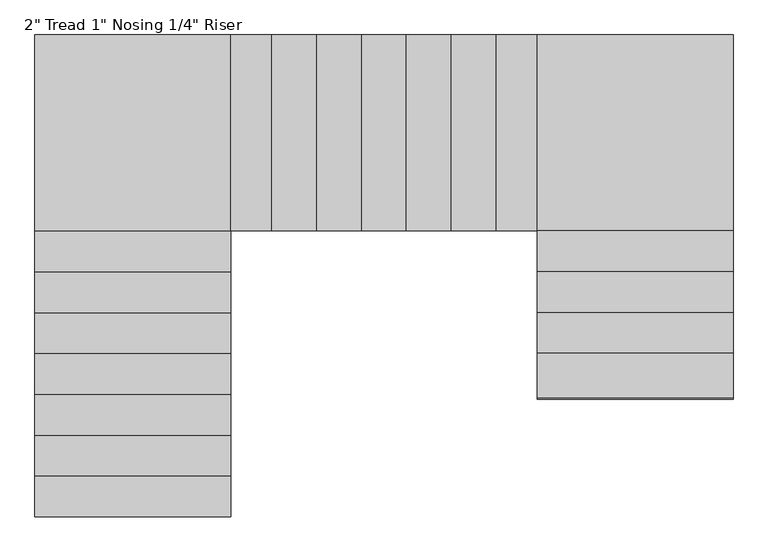
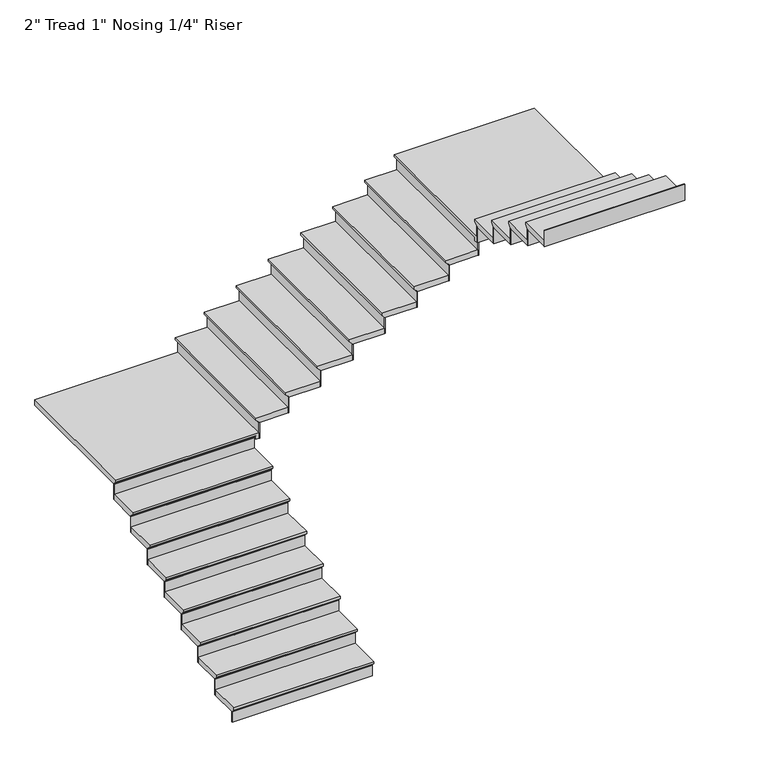
"""IFC4 building model written with IfcOpenShell, lengths in millimetres: stair flight geometry."""

from ifc_helpers import new_model, si_unit, origin, place, context, project, spatial, faceted_brep, source, transform, mapped, element, save


def stair_flight_18be0a75(model_context):
    return source(origin(), model_context, "Body", "Brep", [
        faceted_brep([(14512.1100959, 14647.8480703, 126.0928571), (14512.1100959, 14647.8480703, 145.1428571), (13292.9100959, 14647.8480703, 145.1428571), (13292.9100959, 14647.8480703, 126.0928571), (14512.1100959, 14673.2480703, 100.6928571), (13292.9100959, 14673.2480703, 100.6928571), (14512.1100959, 14927.2480703, 145.1428571), (13292.9100959, 14927.2480703, 145.1428571), (13292.9100959, 14673.2480703, 94.3428571), (13292.9100959, 14927.2480703, 94.3428571), (14512.1100959, 14927.2480703, 94.3428571), (14512.1100959, 14673.2480703, 94.3428571)], [[[0, 1, 2, 3]], [[4, 0, 3, 5]], [[2, 1, 6, 7]], [[8, 9, 10, 11]], [[2, 7, 9, 8, 5, 3]], [[8, 11, 4, 5]], [[6, 1, 0, 4, 11, 10]], [[7, 6, 10, 9]]]),
        faceted_brep([(14512.1100959, 14673.2480703, 94.3428571), (14512.1100959, 14673.2480703, 0.0), (14512.1100959, 14679.5980703, 0.0), (14512.1100959, 14679.5980703, 94.3428571), (13292.9100959, 14673.2480703, 94.3428571), (13292.9100959, 14679.5980703, 94.3428571), (13292.9100959, 14679.5980703, 0.0), (13292.9100959, 14673.2480703, 0.0)], [[[0, 1, 2, 3]], [[4, 5, 6, 7]], [[1, 0, 4, 7]], [[2, 1, 7, 6]], [[3, 2, 6, 5]], [[0, 3, 5, 4]]]),
        faceted_brep([(14512.1100959, 14927.2480703, 239.4857143), (14512.1100959, 14927.2480703, 94.3428571), (14512.1100959, 14933.5980703, 94.3428571), (14512.1100959, 14933.5980703, 239.4857143), (13292.9100959, 14927.2480703, 239.4857143), (13292.9100959, 14933.5980703, 239.4857143), (13292.9100959, 14933.5980703, 94.3428571), (13292.9100959, 14927.2480703, 94.3428571)], [[[0, 1, 2, 3]], [[4, 5, 6, 7]], [[1, 0, 4, 7]], [[2, 1, 7, 6]], [[3, 2, 6, 5]], [[0, 3, 5, 4]]]),
        faceted_brep([(13292.9100959, 14901.8480703, 290.2857143), (14512.1100959, 14901.8480703, 290.2857143), (14512.1100959, 15181.2480703, 290.2857143), (13292.9100959, 15181.2480703, 290.2857143), (13292.9100959, 14927.2480703, 239.4857143), (13292.9100959, 15181.2480703, 239.4857143), (14512.1100959, 15181.2480703, 239.4857143), (14512.1100959, 14927.2480703, 239.4857143), (13292.9100959, 14927.2480703, 245.8357143), (13292.9100959, 14901.8480703, 271.2357143), (14512.1100959, 14927.2480703, 245.8357143), (14512.1100959, 14901.8480703, 271.2357143)], [[[0, 1, 2, 3]], [[4, 5, 6, 7]], [[0, 3, 5, 4, 8, 9]], [[4, 7, 10, 8]], [[2, 1, 11, 10, 7, 6]], [[3, 2, 6, 5]], [[11, 1, 0, 9]], [[10, 11, 9, 8]]]),
        faceted_brep([(14512.1100959, 15181.2480703, 384.6285714), (14512.1100959, 15181.2480703, 239.4857143), (14512.1100959, 15187.5980703, 239.4857143), (14512.1100959, 15187.5980703, 384.6285714), (13292.9100959, 15181.2480703, 384.6285714), (13292.9100959, 15187.5980703, 384.6285714), (13292.9100959, 15187.5980703, 239.4857143), (13292.9100959, 15181.2480703, 239.4857143)], [[[0, 1, 2, 3]], [[4, 5, 6, 7]], [[1, 0, 4, 7]], [[2, 1, 7, 6]], [[3, 2, 6, 5]], [[0, 3, 5, 4]]]),
        faceted_brep([(13292.9100959, 15155.8480703, 435.4285714), (14512.1100959, 15155.8480703, 435.4285714), (14512.1100959, 15435.2480703, 435.4285714), (13292.9100959, 15435.2480703, 435.4285714), (13292.9100959, 15181.2480703, 384.6285714), (13292.9100959, 15435.2480703, 384.6285714), (14512.1100959, 15435.2480703, 384.6285714), (14512.1100959, 15181.2480703, 384.6285714), (13292.9100959, 15181.2480703, 390.9785714), (13292.9100959, 15155.8480703, 416.3785714), (14512.1100959, 15181.2480703, 390.9785714), (14512.1100959, 15155.8480703, 416.3785714)], [[[0, 1, 2, 3]], [[4, 5, 6, 7]], [[0, 3, 5, 4, 8, 9]], [[4, 7, 10, 8]], [[2, 1, 11, 10, 7, 6]], [[3, 2, 6, 5]], [[11, 1, 0, 9]], [[10, 11, 9, 8]]]),
        faceted_brep([(14512.1100959, 15435.2480703, 529.7714286), (14512.1100959, 15435.2480703, 384.6285714), (14512.1100959, 15441.5980703, 384.6285714), (14512.1100959, 15441.5980703, 529.7714286), (13292.9100959, 15435.2480703, 529.7714286), (13292.9100959, 15441.5980703, 529.7714286), (13292.9100959, 15441.5980703, 384.6285714), (13292.9100959, 15435.2480703, 384.6285714)], [[[0, 1, 2, 3]], [[4, 5, 6, 7]], [[1, 0, 4, 7]], [[2, 1, 7, 6]], [[3, 2, 6, 5]], [[0, 3, 5, 4]]]),
        faceted_brep([(13292.9100959, 15409.8480703, 580.5714286), (14512.1100959, 15409.8480703, 580.5714286), (14512.1100959, 15689.2480703, 580.5714286), (13292.9100959, 15689.2480703, 580.5714286), (13292.9100959, 15435.2480703, 529.7714286), (13292.9100959, 15689.2480703, 529.7714286), (14512.1100959, 15689.2480703, 529.7714286), (14512.1100959, 15435.2480703, 529.7714286), (13292.9100959, 15435.2480703, 536.1214286), (13292.9100959, 15409.8480703, 561.5214286), (14512.1100959, 15435.2480703, 536.1214286), (14512.1100959, 15409.8480703, 561.5214286)], [[[0, 1, 2, 3]], [[4, 5, 6, 7]], [[0, 3, 5, 4, 8, 9]], [[4, 7, 10, 8]], [[2, 1, 11, 10, 7, 6]], [[3, 2, 6, 5]], [[11, 1, 0, 9]], [[10, 11, 9, 8]]]),
        faceted_brep([(14512.1100959, 15689.2480703, 674.9142857), (14512.1100959, 15689.2480703, 529.7714286), (14512.1100959, 15695.5980703, 529.7714286), (14512.1100959, 15695.5980703, 674.9142857), (13292.9100959, 15689.2480703, 674.9142857), (13292.9100959, 15695.5980703, 674.9142857), (13292.9100959, 15695.5980703, 529.7714286), (13292.9100959, 15689.2480703, 529.7714286)], [[[0, 1, 2, 3]], [[4, 5, 6, 7]], [[1, 0, 4, 7]], [[2, 1, 7, 6]], [[3, 2, 6, 5]], [[0, 3, 5, 4]]]),
        faceted_brep([(13292.9100959, 15663.8480703, 725.7142857), (14512.1100959, 15663.8480703, 725.7142857), (14512.1100959, 15943.2480703, 725.7142857), (13292.9100959, 15943.2480703, 725.7142857), (13292.9100959, 15689.2480703, 674.9142857), (13292.9100959, 15943.2480703, 674.9142857), (14512.1100959, 15943.2480703, 674.9142857), (14512.1100959, 15689.2480703, 674.9142857), (13292.9100959, 15689.2480703, 681.2642857), (13292.9100959, 15663.8480703, 706.6642857), (14512.1100959, 15689.2480703, 681.2642857), (14512.1100959, 15663.8480703, 706.6642857)], [[[0, 1, 2, 3]], [[4, 5, 6, 7]], [[0, 3, 5, 4, 8, 9]], [[4, 7, 10, 8]], [[2, 1, 11, 10, 7, 6]], [[3, 2, 6, 5]], [[11, 1, 0, 9]], [[10, 11, 9, 8]]]),
        faceted_brep([(14512.1100959, 15943.2480703, 820.0571429), (14512.1100959, 15943.2480703, 674.9142857), (14512.1100959, 15949.5980703, 674.9142857), (14512.1100959, 15949.5980703, 820.0571429), (13292.9100959, 15943.2480703, 820.0571429), (13292.9100959, 15949.5980703, 820.0571429), (13292.9100959, 15949.5980703, 674.9142857), (13292.9100959, 15943.2480703, 674.9142857)], [[[0, 1, 2, 3]], [[4, 5, 6, 7]], [[1, 0, 4, 7]], [[2, 1, 7, 6]], [[3, 2, 6, 5]], [[0, 3, 5, 4]]]),
        faceted_brep([(13292.9100959, 15917.8480703, 870.8571429), (14512.1100959, 15917.8480703, 870.8571429), (14512.1100959, 16197.2480703, 870.8571429), (13292.9100959, 16197.2480703, 870.8571429), (13292.9100959, 15943.2480703, 820.0571429), (13292.9100959, 16197.2480703, 820.0571429), (14512.1100959, 16197.2480703, 820.0571429), (14512.1100959, 15943.2480703, 820.0571429), (13292.9100959, 15943.2480703, 826.4071429), (13292.9100959, 15917.8480703, 851.8071429), (14512.1100959, 15943.2480703, 826.4071429), (14512.1100959, 15917.8480703, 851.8071429)], [[[0, 1, 2, 3]], [[4, 5, 6, 7]], [[0, 3, 5, 4, 8, 9]], [[4, 7, 10, 8]], [[2, 1, 11, 10, 7, 6]], [[3, 2, 6, 5]], [[11, 1, 0, 9]], [[10, 11, 9, 8]]]),
        faceted_brep([(14512.1100959, 16197.2480703, 965.2), (14512.1100959, 16197.2480703, 820.0571429), (14512.1100959, 16203.5980703, 820.0571429), (14512.1100959, 16203.5980703, 965.2), (13292.9100959, 16197.2480703, 965.2), (13292.9100959, 16203.5980703, 965.2), (13292.9100959, 16203.5980703, 820.0571429), (13292.9100959, 16197.2480703, 820.0571429)], [[[0, 1, 2, 3]], [[4, 5, 6, 7]], [[1, 0, 4, 7]], [[2, 1, 7, 6]], [[3, 2, 6, 5]], [[0, 3, 5, 4]]]),
        faceted_brep([(13292.9100959, 16171.8480703, 1016.0), (14512.1100959, 16171.8480703, 1016.0), (14512.1100959, 16451.2480703, 1016.0), (13292.9100959, 16451.2480703, 1016.0), (13292.9100959, 16197.2480703, 965.2), (13292.9100959, 16451.2480703, 965.2), (14512.1100959, 16451.2480703, 965.2), (14512.1100959, 16197.2480703, 965.2), (13292.9100959, 16197.2480703, 971.55), (13292.9100959, 16171.8480703, 996.95), (14512.1100959, 16197.2480703, 971.55), (14512.1100959, 16171.8480703, 996.95)], [[[0, 1, 2, 3]], [[4, 5, 6, 7]], [[0, 3, 5, 4, 8, 9]], [[4, 7, 10, 8]], [[2, 1, 11, 10, 7, 6]], [[3, 2, 6, 5]], [[11, 1, 0, 9]], [[10, 11, 9, 8]]]),
        faceted_brep([(14512.1100959, 16451.2480703, 1110.3428571), (14512.1100959, 16451.2480703, 965.2), (14512.1100959, 16457.5980703, 965.2), (14512.1100959, 16457.5980703, 1110.3428571), (13292.9100959, 16451.2480703, 1110.3428571), (13292.9100959, 16457.5980703, 1110.3428571), (13292.9100959, 16457.5980703, 965.2), (13292.9100959, 16451.2480703, 965.2)], [[[0, 1, 2, 3]], [[4, 5, 6, 7]], [[1, 0, 4, 7]], [[2, 1, 7, 6]], [[3, 2, 6, 5]], [[0, 3, 5, 4]]]),
        faceted_brep([(14537.5100959, 17645.0480703, 1161.1428571), (13292.9100959, 17645.0480703, 1161.1428571), (13292.9100959, 16425.8480703, 1161.1428571), (14537.5100959, 16425.8480703, 1161.1428571), (13292.9100959, 17645.0480703, 1110.3428571), (14537.5100959, 17645.0480703, 1110.3428571), (14537.5100959, 16425.8480703, 1110.3428571), (14512.1100959, 16425.8480703, 1110.3428571), (14512.1100959, 16451.2480703, 1110.3428571), (13292.9100959, 16451.2480703, 1110.3428571), (13292.9100959, 16451.2480703, 1116.6928571), (13292.9100959, 16425.8480703, 1142.0928571), (14512.1100959, 16451.2480703, 1116.6928571), (14512.1100959, 16425.8480703, 1142.0928571)], [[[0, 1, 2, 3]], [[4, 5, 6, 7, 8, 9]], [[1, 0, 5, 4]], [[2, 1, 4, 9, 10, 11]], [[9, 8, 12, 10]], [[8, 7, 13, 12]], [[3, 2, 11, 13, 7, 6]], [[0, 3, 6, 5]], [[11, 10, 12, 13]]]),
        faceted_brep([(14537.5100959, 16425.8480703, 1255.4857143), (14537.5100959, 16425.8480703, 1110.3428571), (14543.8600959, 16425.8480703, 1110.3428571), (14543.8600959, 16425.8480703, 1255.4857143), (14537.5100959, 17645.0480703, 1255.4857143), (14543.8600959, 17645.0480703, 1255.4857143), (14543.8600959, 17645.0480703, 1110.3428571), (14537.5100959, 17645.0480703, 1110.3428571)], [[[0, 1, 2, 3]], [[4, 5, 6, 7]], [[1, 0, 4, 7]], [[2, 1, 7, 6]], [[3, 2, 6, 5]], [[0, 3, 5, 4]]]),
        faceted_brep([(14512.1100959, 17645.0480703, 1306.2857143), (14512.1100959, 16425.8480703, 1306.2857143), (14791.5100959, 16425.8480703, 1306.2857143), (14791.5100959, 17645.0480703, 1306.2857143), (14537.5100959, 17645.0480703, 1255.4857143), (14791.5100959, 17645.0480703, 1255.4857143), (14791.5100959, 16425.8480703, 1255.4857143), (14537.5100959, 16425.8480703, 1255.4857143), (14537.5100959, 17645.0480703, 1261.8357143), (14512.1100959, 17645.0480703, 1287.2357143), (14537.5100959, 16425.8480703, 1261.8357143), (14512.1100959, 16425.8480703, 1287.2357143)], [[[0, 1, 2, 3]], [[4, 5, 6, 7]], [[0, 3, 5, 4, 8, 9]], [[4, 7, 10, 8]], [[2, 1, 11, 10, 7, 6]], [[3, 2, 6, 5]], [[11, 1, 0, 9]], [[10, 11, 9, 8]]]),
        faceted_brep([(14791.5100959, 16425.8480703, 1400.6285714), (14791.5100959, 16425.8480703, 1255.4857143), (14797.8600959, 16425.8480703, 1255.4857143), (14797.8600959, 16425.8480703, 1400.6285714), (14791.5100959, 17645.0480703, 1400.6285714), (14797.8600959, 17645.0480703, 1400.6285714), (14797.8600959, 17645.0480703, 1255.4857143), (14791.5100959, 17645.0480703, 1255.4857143)], [[[0, 1, 2, 3]], [[4, 5, 6, 7]], [[1, 0, 4, 7]], [[2, 1, 7, 6]], [[3, 2, 6, 5]], [[0, 3, 5, 4]]]),
        faceted_brep([(14766.1100959, 17645.0480703, 1451.4285714), (14766.1100959, 16425.8480703, 1451.4285714), (15070.9100959, 16425.8480703, 1451.4285714), (15070.9100959, 17645.0480703, 1451.4285714), (14791.5100959, 17645.0480703, 1400.6285714), (15070.9100959, 17645.0480703, 1400.6285714), (15070.9100959, 16425.8480703, 1400.6285714), (14791.5100959, 16425.8480703, 1400.6285714), (14791.5100959, 17645.0480703, 1406.9785714), (14766.1100959, 17645.0480703, 1432.3785714), (14791.5100959, 16425.8480703, 1406.9785714), (14766.1100959, 16425.8480703, 1432.3785714)], [[[0, 1, 2, 3]], [[4, 5, 6, 7]], [[0, 3, 5, 4, 8, 9]], [[4, 7, 10, 8]], [[2, 1, 11, 10, 7, 6]], [[3, 2, 6, 5]], [[11, 1, 0, 9]], [[10, 11, 9, 8]]]),
        faceted_brep([(15070.9100959, 16425.8480703, 1545.7714286), (15070.9100959, 16425.8480703, 1400.6285714), (15077.2600959, 16425.8480703, 1400.6285714), (15077.2600959, 16425.8480703, 1545.7714286), (15070.9100959, 17645.0480703, 1545.7714286), (15077.2600959, 17645.0480703, 1545.7714286), (15077.2600959, 17645.0480703, 1400.6285714), (15070.9100959, 17645.0480703, 1400.6285714)], [[[0, 1, 2, 3]], [[4, 5, 6, 7]], [[1, 0, 4, 7]], [[2, 1, 7, 6]], [[3, 2, 6, 5]], [[0, 3, 5, 4]]]),
        faceted_brep([(15045.5100959, 17645.0480703, 1596.5714286), (15045.5100959, 16425.8480703, 1596.5714286), (15350.3100959, 16425.8480703, 1596.5714286), (15350.3100959, 17645.0480703, 1596.5714286), (15070.9100959, 17645.0480703, 1545.7714286), (15350.3100959, 17645.0480703, 1545.7714286), (15350.3100959, 16425.8480703, 1545.7714286), (15070.9100959, 16425.8480703, 1545.7714286), (15070.9100959, 17645.0480703, 1552.1214286), (15045.5100959, 17645.0480703, 1577.5214286), (15070.9100959, 16425.8480703, 1552.1214286), (15045.5100959, 16425.8480703, 1577.5214286)], [[[0, 1, 2, 3]], [[4, 5, 6, 7]], [[0, 3, 5, 4, 8, 9]], [[4, 7, 10, 8]], [[2, 1, 11, 10, 7, 6]], [[3, 2, 6, 5]], [[11, 1, 0, 9]], [[10, 11, 9, 8]]]),
        faceted_brep([(15350.3100959, 16425.8480703, 1690.9142857), (15350.3100959, 16425.8480703, 1545.7714286), (15356.6600959, 16425.8480703, 1545.7714286), (15356.6600959, 16425.8480703, 1690.9142857), (15350.3100959, 17645.0480703, 1690.9142857), (15356.6600959, 17645.0480703, 1690.9142857), (15356.6600959, 17645.0480703, 1545.7714286), (15350.3100959, 17645.0480703, 1545.7714286)], [[[0, 1, 2, 3]], [[4, 5, 6, 7]], [[1, 0, 4, 7]], [[2, 1, 7, 6]], [[3, 2, 6, 5]], [[0, 3, 5, 4]]]),
        faceted_brep([(15324.9100959, 17645.0480703, 1741.7142857), (15324.9100959, 16425.8480703, 1741.7142857), (15629.7100959, 16425.8480703, 1741.7142857), (15629.7100959, 17645.0480703, 1741.7142857), (15350.3100959, 17645.0480703, 1690.9142857), (15629.7100959, 17645.0480703, 1690.9142857), (15629.7100959, 16425.8480703, 1690.9142857), (15350.3100959, 16425.8480703, 1690.9142857), (15350.3100959, 17645.0480703, 1697.2642857), (15324.9100959, 17645.0480703, 1722.6642857), (15350.3100959, 16425.8480703, 1697.2642857), (15324.9100959, 16425.8480703, 1722.6642857)], [[[0, 1, 2, 3]], [[4, 5, 6, 7]], [[0, 3, 5, 4, 8, 9]], [[4, 7, 10, 8]], [[2, 1, 11, 10, 7, 6]], [[3, 2, 6, 5]], [[11, 1, 0, 9]], [[10, 11, 9, 8]]]),
        faceted_brep([(15629.7100959, 16425.8480703, 1836.0571429), (15629.7100959, 16425.8480703, 1690.9142857), (15636.0600959, 16425.8480703, 1690.9142857), (15636.0600959, 16425.8480703, 1836.0571429), (15629.7100959, 17645.0480703, 1836.0571429), (15636.0600959, 17645.0480703, 1836.0571429), (15636.0600959, 17645.0480703, 1690.9142857), (15629.7100959, 17645.0480703, 1690.9142857)], [[[0, 1, 2, 3]], [[4, 5, 6, 7]], [[1, 0, 4, 7]], [[2, 1, 7, 6]], [[3, 2, 6, 5]], [[0, 3, 5, 4]]]),
        faceted_brep([(15604.3100959, 17645.0480703, 1886.8571429), (15604.3100959, 16425.8480703, 1886.8571429), (15909.1100959, 16425.8480703, 1886.8571429), (15909.1100959, 17645.0480703, 1886.8571429), (15629.7100959, 17645.0480703, 1836.0571429), (15909.1100959, 17645.0480703, 1836.0571429), (15909.1100959, 16425.8480703, 1836.0571429), (15629.7100959, 16425.8480703, 1836.0571429), (15629.7100959, 17645.0480703, 1842.4071429), (15604.3100959, 17645.0480703, 1867.8071429), (15629.7100959, 16425.8480703, 1842.4071429), (15604.3100959, 16425.8480703, 1867.8071429)], [[[0, 1, 2, 3]], [[4, 5, 6, 7]], [[0, 3, 5, 4, 8, 9]], [[4, 7, 10, 8]], [[2, 1, 11, 10, 7, 6]], [[3, 2, 6, 5]], [[11, 1, 0, 9]], [[10, 11, 9, 8]]]),
        faceted_brep([(15909.1100959, 16425.8480703, 1981.2), (15909.1100959, 16425.8480703, 1836.0571429), (15915.4600959, 16425.8480703, 1836.0571429), (15915.4600959, 16425.8480703, 1981.2), (15909.1100959, 17645.0480703, 1981.2), (15915.4600959, 17645.0480703, 1981.2), (15915.4600959, 17645.0480703, 1836.0571429), (15909.1100959, 17645.0480703, 1836.0571429)], [[[0, 1, 2, 3]], [[4, 5, 6, 7]], [[1, 0, 4, 7]], [[2, 1, 7, 6]], [[3, 2, 6, 5]], [[0, 3, 5, 4]]]),
        faceted_brep([(15883.7100959, 17645.0480703, 2032.0), (15883.7100959, 16425.8480703, 2032.0), (16188.5100959, 16425.8480703, 2032.0), (16188.5100959, 17645.0480703, 2032.0), (15909.1100959, 17645.0480703, 1981.2), (16188.5100959, 17645.0480703, 1981.2), (16188.5100959, 16425.8480703, 1981.2), (15909.1100959, 16425.8480703, 1981.2), (15909.1100959, 17645.0480703, 1987.55), (15883.7100959, 17645.0480703, 2012.95), (15909.1100959, 16425.8480703, 1987.55), (15883.7100959, 16425.8480703, 2012.95)], [[[0, 1, 2, 3]], [[4, 5, 6, 7]], [[0, 3, 5, 4, 8, 9]], [[4, 7, 10, 8]], [[2, 1, 11, 10, 7, 6]], [[3, 2, 6, 5]], [[11, 1, 0, 9]], [[10, 11, 9, 8]]]),
        faceted_brep([(16188.5100959, 16425.8480703, 2126.3428571), (16188.5100959, 16425.8480703, 1981.2), (16194.8600959, 16425.8480703, 1981.2), (16194.8600959, 16425.8480703, 2126.3428571), (16188.5100959, 17645.0480703, 2126.3428571), (16194.8600959, 17645.0480703, 2126.3428571), (16194.8600959, 17645.0480703, 1981.2), (16188.5100959, 17645.0480703, 1981.2)], [[[0, 1, 2, 3]], [[4, 5, 6, 7]], [[1, 0, 4, 7]], [[2, 1, 7, 6]], [[3, 2, 6, 5]], [[0, 3, 5, 4]]]),
        faceted_brep([(16163.1100959, 17645.0480703, 2177.1428571), (16163.1100959, 16425.8480703, 2177.1428571), (16442.5100959, 16425.8480703, 2177.1428571), (16442.5100959, 17645.0480703, 2177.1428571), (16188.5100959, 17645.0480703, 2126.3428571), (16442.5100959, 17645.0480703, 2126.3428571), (16442.5100959, 16425.8480703, 2126.3428571), (16188.5100959, 16425.8480703, 2126.3428571), (16188.5100959, 17645.0480703, 2132.6928571), (16163.1100959, 17645.0480703, 2158.0928571), (16188.5100959, 16425.8480703, 2132.6928571), (16163.1100959, 16425.8480703, 2158.0928571)], [[[0, 1, 2, 3]], [[4, 5, 6, 7]], [[0, 3, 5, 4, 8, 9]], [[4, 7, 10, 8]], [[2, 1, 11, 10, 7, 6]], [[3, 2, 6, 5]], [[11, 1, 0, 9]], [[10, 11, 9, 8]]]),
        faceted_brep([(16442.5100959, 16425.8480703, 2271.4857143), (16442.5100959, 16425.8480703, 2126.3428571), (16448.8600959, 16425.8480703, 2126.3428571), (16448.8600959, 16425.8480703, 2271.4857143), (16442.5100959, 17645.0480703, 2271.4857143), (16448.8600959, 17645.0480703, 2271.4857143), (16448.8600959, 17645.0480703, 2126.3428571), (16442.5100959, 17645.0480703, 2126.3428571)], [[[0, 1, 2, 3]], [[4, 5, 6, 7]], [[1, 0, 4, 7]], [[2, 1, 7, 6]], [[3, 2, 6, 5]], [[0, 3, 5, 4]]]),
        faceted_brep([(17636.3100959, 16400.4480703, 2322.2857143), (17636.3100959, 17645.0480703, 2322.2857143), (16417.1100959, 17645.0480703, 2322.2857143), (16417.1100959, 16400.4480703, 2322.2857143), (17636.3100959, 17645.0480703, 2271.4857143), (17636.3100959, 16400.4480703, 2271.4857143), (16417.1100959, 16400.4480703, 2271.4857143), (16417.1100959, 16425.8480703, 2271.4857143), (16442.5100959, 16425.8480703, 2271.4857143), (16442.5100959, 17645.0480703, 2271.4857143), (16442.5100959, 17645.0480703, 2277.8357143), (16417.1100959, 17645.0480703, 2303.2357143), (16442.5100959, 16425.8480703, 2277.8357143), (16417.1100959, 16425.8480703, 2303.2357143)], [[[0, 1, 2, 3]], [[4, 5, 6, 7, 8, 9]], [[1, 0, 5, 4]], [[2, 1, 4, 9, 10, 11]], [[9, 8, 12, 10]], [[8, 7, 13, 12]], [[3, 2, 11, 13, 7, 6]], [[0, 3, 6, 5]], [[11, 10, 12, 13]]]),
        faceted_brep([(16417.1100959, 16400.4480703, 2416.6285714), (16417.1100959, 16400.4480703, 2271.4857143), (16417.1100959, 16394.0980703, 2271.4857143), (16417.1100959, 16394.0980703, 2416.6285714), (17636.3100959, 16400.4480703, 2416.6285714), (17636.3100959, 16394.0980703, 2416.6285714), (17636.3100959, 16394.0980703, 2271.4857143), (17636.3100959, 16400.4480703, 2271.4857143)], [[[0, 1, 2, 3]], [[4, 5, 6, 7]], [[1, 0, 4, 7]], [[2, 1, 7, 6]], [[3, 2, 6, 5]], [[0, 3, 5, 4]]]),
        faceted_brep([(17636.3100959, 16425.8480703, 2467.4285714), (16417.1100959, 16425.8480703, 2467.4285714), (16417.1100959, 16146.4480703, 2467.4285714), (17636.3100959, 16146.4480703, 2467.4285714), (17636.3100959, 16400.4480703, 2416.6285714), (17636.3100959, 16146.4480703, 2416.6285714), (16417.1100959, 16146.4480703, 2416.6285714), (16417.1100959, 16400.4480703, 2416.6285714), (17636.3100959, 16400.4480703, 2422.9785714), (17636.3100959, 16425.8480703, 2448.3785714), (16417.1100959, 16400.4480703, 2422.9785714), (16417.1100959, 16425.8480703, 2448.3785714)], [[[0, 1, 2, 3]], [[4, 5, 6, 7]], [[0, 3, 5, 4, 8, 9]], [[4, 7, 10, 8]], [[2, 1, 11, 10, 7, 6]], [[3, 2, 6, 5]], [[11, 1, 0, 9]], [[10, 11, 9, 8]]]),
        faceted_brep([(16417.1100959, 16146.4480703, 2561.7714286), (16417.1100959, 16146.4480703, 2416.6285714), (16417.1100959, 16140.0980703, 2416.6285714), (16417.1100959, 16140.0980703, 2561.7714286), (17636.3100959, 16146.4480703, 2561.7714286), (17636.3100959, 16140.0980703, 2561.7714286), (17636.3100959, 16140.0980703, 2416.6285714), (17636.3100959, 16146.4480703, 2416.6285714)], [[[0, 1, 2, 3]], [[4, 5, 6, 7]], [[1, 0, 4, 7]], [[2, 1, 7, 6]], [[3, 2, 6, 5]], [[0, 3, 5, 4]]]),
        faceted_brep([(17636.3100959, 16171.8480703, 2612.5714286), (16417.1100959, 16171.8480703, 2612.5714286), (16417.1100959, 15892.4480703, 2612.5714286), (17636.3100959, 15892.4480703, 2612.5714286), (17636.3100959, 16146.4480703, 2561.7714286), (17636.3100959, 15892.4480703, 2561.7714286), (16417.1100959, 15892.4480703, 2561.7714286), (16417.1100959, 16146.4480703, 2561.7714286), (17636.3100959, 16146.4480703, 2568.1214286), (17636.3100959, 16171.8480703, 2593.5214286), (16417.1100959, 16146.4480703, 2568.1214286), (16417.1100959, 16171.8480703, 2593.5214286)], [[[0, 1, 2, 3]], [[4, 5, 6, 7]], [[0, 3, 5, 4, 8, 9]], [[4, 7, 10, 8]], [[2, 1, 11, 10, 7, 6]], [[3, 2, 6, 5]], [[11, 1, 0, 9]], [[10, 11, 9, 8]]]),
        faceted_brep([(16417.1100959, 15892.4480703, 2706.9142857), (16417.1100959, 15892.4480703, 2561.7714286), (16417.1100959, 15886.0980703, 2561.7714286), (16417.1100959, 15886.0980703, 2706.9142857), (17636.3100959, 15892.4480703, 2706.9142857), (17636.3100959, 15886.0980703, 2706.9142857), (17636.3100959, 15886.0980703, 2561.7714286), (17636.3100959, 15892.4480703, 2561.7714286)], [[[0, 1, 2, 3]], [[4, 5, 6, 7]], [[1, 0, 4, 7]], [[2, 1, 7, 6]], [[3, 2, 6, 5]], [[0, 3, 5, 4]]]),
        faceted_brep([(17636.3100959, 15917.8480703, 2757.7142857), (16417.1100959, 15917.8480703, 2757.7142857), (16417.1100959, 15638.4480703, 2757.7142857), (17636.3100959, 15638.4480703, 2757.7142857), (17636.3100959, 15892.4480703, 2706.9142857), (17636.3100959, 15638.4480703, 2706.9142857), (16417.1100959, 15638.4480703, 2706.9142857), (16417.1100959, 15892.4480703, 2706.9142857), (17636.3100959, 15892.4480703, 2713.2642857), (17636.3100959, 15917.8480703, 2738.6642857), (16417.1100959, 15892.4480703, 2713.2642857), (16417.1100959, 15917.8480703, 2738.6642857)], [[[0, 1, 2, 3]], [[4, 5, 6, 7]], [[0, 3, 5, 4, 8, 9]], [[4, 7, 10, 8]], [[2, 1, 11, 10, 7, 6]], [[3, 2, 6, 5]], [[11, 1, 0, 9]], [[10, 11, 9, 8]]]),
        faceted_brep([(16417.1100959, 15638.4480703, 2852.0571429), (16417.1100959, 15638.4480703, 2706.9142857), (16417.1100959, 15632.0980703, 2706.9142857), (16417.1100959, 15632.0980703, 2852.0571429), (17636.3100959, 15638.4480703, 2852.0571429), (17636.3100959, 15632.0980703, 2852.0571429), (17636.3100959, 15632.0980703, 2706.9142857), (17636.3100959, 15638.4480703, 2706.9142857)], [[[0, 1, 2, 3]], [[4, 5, 6, 7]], [[1, 0, 4, 7]], [[2, 1, 7, 6]], [[3, 2, 6, 5]], [[0, 3, 5, 4]]]),
        faceted_brep([(16417.1100959, 15384.4480703, 2997.2), (16417.1100959, 15384.4480703, 2852.0571429), (16417.1100959, 15378.0980703, 2852.0571429), (16417.1100959, 15378.0980703, 2997.2), (17636.3100959, 15384.4480703, 2997.2), (17636.3100959, 15378.0980703, 2997.2), (17636.3100959, 15378.0980703, 2852.0571429), (17636.3100959, 15384.4480703, 2852.0571429)], [[[0, 1, 2, 3]], [[4, 5, 6, 7]], [[1, 0, 4, 7]], [[2, 1, 7, 6]], [[3, 2, 6, 5]], [[0, 3, 5, 4]]]),
        faceted_brep([(17636.3100959, 15663.8480703, 2902.8571429), (16417.1100959, 15663.8480703, 2902.8571429), (16417.1100959, 15384.4480703, 2902.8571429), (17636.3100959, 15384.4480703, 2902.8571429), (17636.3100959, 15638.4480703, 2852.0571429), (17636.3100959, 15384.4480703, 2852.0571429), (16417.1100959, 15384.4480703, 2852.0571429), (16417.1100959, 15638.4480703, 2852.0571429), (17636.3100959, 15638.4480703, 2858.4071429), (17636.3100959, 15663.8480703, 2883.8071429), (16417.1100959, 15638.4480703, 2858.4071429), (16417.1100959, 15663.8480703, 2883.8071429)], [[[0, 1, 2, 3]], [[4, 5, 6, 7]], [[0, 3, 5, 4, 8, 9]], [[4, 7, 10, 8]], [[2, 1, 11, 10, 7, 6]], [[3, 2, 6, 5]], [[11, 1, 0, 9]], [[10, 11, 9, 8]]]),
    ])


if __name__ == "__main__":
    model = new_model("IFC4")
    model_context = context("Model", 3, world=origin())
    ifc_project = project(units=[si_unit("LENGTHUNIT", "METRE", prefix="MILLI")], contexts=[model_context])
    site = spatial("IfcSite", under=ifc_project)
    building = spatial("IfcBuilding", under=site)
    placement = place(None, origin())
    stair_flight_shape = stair_flight_18be0a75(model_context)
    element("IfcStairFlight", 1, ObjectType="2\" Tread 1\" Nosing 1/4\" Riser", at=placement, inside=building, context=model_context, shape_type="MappedRepresentation", body=[
        mapped(stair_flight_shape, transform((0.0, 0.0, 0.0), x_axis=(1.0, 0.0, 0.0), y_axis=(0.0, 1.0, 0.0), z_axis=(0.0, 0.0, 1.0))),
    ])
    save(model, "model.ifc")
